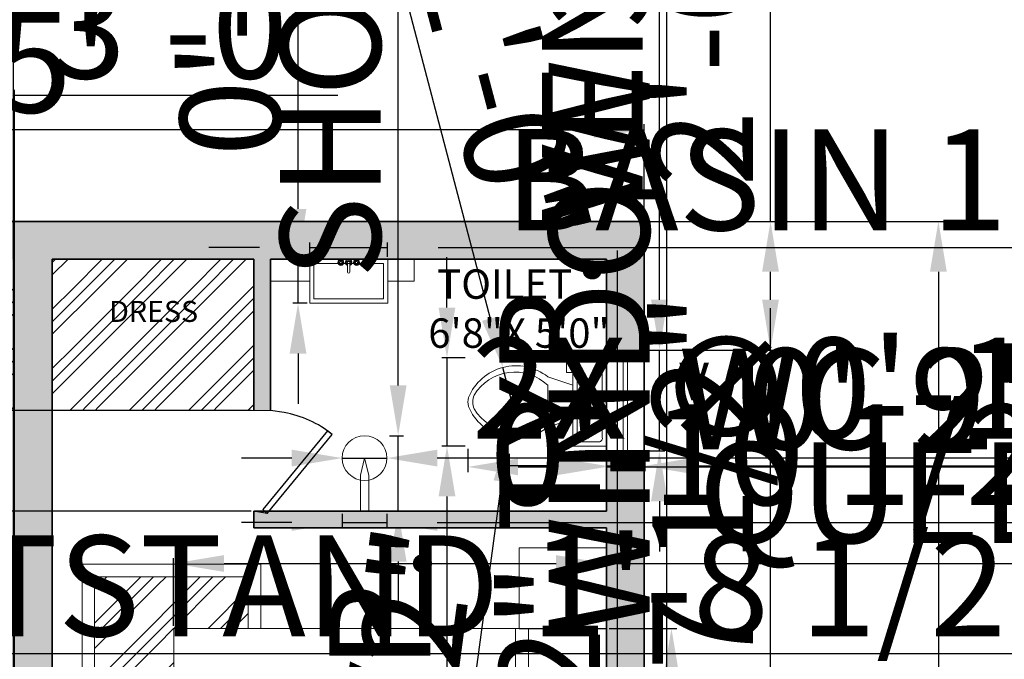
# Model space of a CAD drawing. Units: inches. Extents: x 830 to 1639, y 2591 to 3595.
# Tile 5 of 7: x 1133 to 1367, y 3108 to 3260. Entities that reach past the tile are written whole.
import ezdxf

# ---------------------------------------------------------------- set-up
doc = ezdxf.new("R2010")
doc.units = ezdxf.units.IN
doc.layers.get('0').update_dxf_attribs({"color": 250})
for name, color, linetype, lineweight in [('A-ANNO-DIMS', 2, 'Continuous', 18), ('A-ANNO-TEXT', 7, 'Continuous', 18), ('A-AREA-IDEN', 7, 'Continuous', 25), ('A-DOOR', 3, 'Continuous', 25), ('A-FLOR-CASE', 8, 'Continuous', 18), ('A-FLOR-FIXT', 8, 'Continuous', 18), ('A-FLOR-PATT', 252, 'Continuous', 13), ('A-FURN', 8, 'Continuous', 18), ('A-GLAZ', 4, 'Continuous', 18), ('A-WALL', 7, 'Continuous', 35), ('A-WALL-PATT', 5, 'Continuous', 13), ('C-PROP', 7, 'Continuous', 35)]:
    doc.layers.add(name, color=color, linetype=linetype, lineweight=lineweight)
doc.styles.get("Standard").update_dxf_attribs({"font": 'arial.ttf'})
doc.dimstyles.new('ISO-25', dxfattribs={"dimtxt": 24, "dimasz": 12, "dimexe": 1.25, "dimexo": 0.625, "dimtad": 1, "dimdec": 0, "dimlunit": 3, "dimtxsty": 'Standard', "dimcen": 2.5, "dimadec": 0, "dimazin": 0, "dimtfac": 1, "dimtdec": 0, "dimtmove": 0, "dimatfit": 3, "dimfxl": 1, "dimarcsym": 0})

# ---------------------------------------------------------------- blocks, each defined once
blk = doc.blocks.new('Toilet - top')
for p, q in [((9.5, -6), (9.5, -2)), ((-10, -8.5), (-8, -8.5)), ((-10, -9.5), (-10, -8.5)), ((-8, -8.5), (-8, -8)), ((-7, -8), (-7, -9.5)), ((-4, -8), (-6, -14)), ((4, -8), (6, -14)), ((-7, -9.5), (-10, -9.5)), ((4, -14), (-4, -14))]:
    blk.add_line(p, q)
blk.add_lwpolyline([(10.5, -8), (10.5, 0), (-10.5, 0), (-10.5, -8)], close=True)
for points in [[(-9.5, -2), (-9.5, -6)], [(8.5, -1), (-8.5, -1)], [(-8.5, -7), (8.5, -7)]]:
    blk.add_lwpolyline(points)
for centre, radius, start, end in [((-8.62, -1.88), 0.884, 81.8699, 188.1301), ((8.62, -1.88), 0.884, 351.8699, 98.1301), ((-8.62, -6.12), 0.884, 171.8699, 278.1301), ((8.62, -6.12), 0.884, 261.8699, 8.1301), ((3.52, -21.58), 12.17, 141.4691, 247.9714), ((4.2, -21.82), 11.33, 136.3677, 238.9468), ((-3.52, -21.58), 12.17, 292.0284, 38.5307), ((-4.2, -21.82), 11.33, 301.053, 43.6321), ((0, -27.88), 4, 245.7318, 294.2682), ((0, -29), 4, 254.8605, 285.1395)]:
    blk.add_arc(centre, radius, start, end)
blk = doc.blocks.new('*U9')
for p, q in [((-750, 0), (-750, -100)), ((0, 0), (0, -100))]:
    blk.add_line(p, q)
blk.add_lwpolyline([(0, 0), (-649.5, 375), (-671.4, 337.1), (-21.9, -37.9)], close=True)
blk.add_arc((0, 0), 750, 150, 180)
blk = doc.blocks.new('Faucet - Bathroom top')
for p, q in [((-4.107, 0.125), (-4.375, 0.125)), ((-3.75, 0.4788), (-3.75, 0.75)), ((-3.5, 0.482), (-3.5, 0.75)), ((-3.1461, 0.125), (-2.875, 0.125)), ((3.143, 0.125), (2.875, 0.125)), ((3.5, 0.4788), (3.5, 0.75)), ((3.75, 0.482), (3.75, 0.75)), ((4.1039, 0.125), (4.375, 0.125)), ((-4.1039, -0.125), (-4.375, -0.125)), ((-3.75, -0.4821), (-3.75, -0.75)), ((-3.5, -0.4789), (-3.5, -0.75)), ((-3.143, -0.125), (-2.875, -0.125)), ((-0.5, -0.8639), (-0.5, -4.5)), ((0.5, -4.5), (0.5, -0.8631)), ((3.1461, -0.125), (2.875, -0.125)), ((3.5, -0.4821), (3.5, -0.75)), ((3.75, -0.4789), (3.75, -0.75)), ((4.107, -0.125), (4.375, -0.125))]:
    blk.add_line(p, q)
for centre, radius in [((-3.625, 0), 1.375), ((-4.625, 0), 0.2795), ((-3.625, 0), 0.5), ((-3.625, 1), 0.2795), ((-2.625, 0), 0.2795), ((0, 0), 0.5), ((3.625, 0), 1.375), ((2.625, 0), 0.2795), ((3.625, 0), 0.5), ((3.625, 1), 0.2795), ((4.625, 0), 0.2795), ((-3.625, -1), 0.2795), ((3.625, -1), 0.2795)]:
    blk.add_circle(centre, radius)
for centre, radius, start, end in [((-3.625, 0), 1, 105.2407, 164.2093), ((-3.625, 0), 1, 16.44125, 74.07887), ((0, 0), 1.5, 289.6514, 250.3603), ((0, 0), 1, 300.3431, 239.7554), ((3.625, 0), 1, 106.12, 164.0884), ((3.625, 0), 1, 16.23422, 73.90469), ((-3.625, 0), 1, 196.2342, 253.9047), ((-3.625, 0), 1, 286.12, 344.0884), ((0, -4.5), 0.5, 180, 0), ((3.625, 0), 1, 196.4413, 254.0789), ((3.625, 0), 1, 285.2407, 344.2093)]:
    blk.add_arc(centre, radius, start, end)
blk = doc.blocks.new('Bed - Queen')
for p, q in [((0, -80.00003), (0, 0)), ((0, 0), (59.99999, 0)), ((59.99999, 0), (59.99999, -80.00003)), ((7.99999, -1.2), (28.79998, -1.2)), ((7.99999, -14.4), (7.99999, -1.2)), ((28.79998, -1.2), (28.79998, -14.4)), ((31.19999, -1.2), (51.99999, -1.2)), ((31.19999, -14.4), (31.19999, -1.2)), ((51.99999, -1.2), (51.99999, -16.4)), ((0, -14.4), (44.8, -14.4)), ((59.99999, -29.6), (44.8, -14.4)), ((44.8, -14.4), (44.8, -29.6)), ((44.8, -16.8), (0, -16.8)), ((51.99999, -16.4), (46.79936, -16.4)), ((44.8, -29.6), (59.99999, -29.6)), ((59.99999, -80.00003), (0, -80.00003))]:
    blk.add_line(p, q)
blk = doc.blocks.new('*D14')
at = {"layer": 'A-ANNO-DIMS', "color": 0, "lineweight": -2, "transparency": 16777216}
for p, q in [((1282.21, 3212.09), (1352.88, 3212.09)), ((1351.63, 3200.09), (1351.63, 2684.09)), ((1282.21, 2672.09), (1352.88, 2672.09))]:
    blk.add_line(p, q, dxfattribs=at)
at = {"layer": 'A-ANNO-DIMS', "color": 0, "transparency": 16777216}
for points in [[(1349.63, 3200.09), (1353.63, 3200.09), (1351.63, 3212.09)], [(1349.63, 2684.09), (1353.63, 2684.09), (1351.63, 2672.09)]]:
    blk.add_solid(points, dxfattribs=at)
at = {"layer": 'Defpoints', "color": 0, "transparency": 16777216}
for p in [(1281.59, 3212.09), (1281.59, 2672.09), (1351.63, 2672.09)]:
    blk.add_point(p, dxfattribs=at)
at = {"layer": 'A-ANNO-DIMS', "color": 0, "transparency": 16777216, "insert": (1338.8, 2942.09), "char_height": 24, "attachment_point": 5, "rotation": 90}
blk.add_mtext("45'", dxfattribs=at)
blk = doc.blocks.new('*D15')
at = {"layer": 'A-ANNO-DIMS', "color": 0, "lineweight": -2, "transparency": 16777216}
for p, q in [((981.59, 3212.71), (981.59, 3235.25)), ((993.59, 3234), (1269.59, 3234)), ((1281.59, 3212.71), (1281.59, 3235.25))]:
    blk.add_line(p, q, dxfattribs=at)
at = {"layer": 'A-ANNO-DIMS', "color": 0, "transparency": 16777216}
for points in [[(993.59, 3236), (993.59, 3232), (981.59, 3234)], [(1269.59, 3236), (1269.59, 3232), (1281.59, 3234)]]:
    blk.add_solid(points, dxfattribs=at)
at = {"layer": 'Defpoints', "color": 0, "transparency": 16777216}
for p in [(1281.59, 3234), (981.59, 3212.09), (1281.59, 3212.09)]:
    blk.add_point(p, dxfattribs=at)
at = {"layer": 'A-ANNO-DIMS', "color": 0, "transparency": 16777216, "insert": (1131.59, 3246.88), "char_height": 24, "attachment_point": 5}
blk.add_mtext("25'", dxfattribs=at)
blk = doc.blocks.new('VENT-24IN')
for p, q in [((0, 24), (9, 24)), ((0, 0), (0, 24)), ((4, 0), (4, 24)), ((5, 24), (5, 0)), ((9, 24), (9, 0)), ((9, 0), (0, 0))]:
    blk.add_line(p, q)
blk = doc.blocks.new('BEDSIDE-TABLE')
blk.add_lwpolyline([(20.72, 0), (0, 0), (0, 19.25), (20.72, 19.25)], close=True)
blk = doc.blocks.new('LAVATORY-RECT')
for points in [[(0, 10.45), (18.57, 10.45), (18.57, 0), (0, 0)], [(1, 9.45), (17.57, 9.45), (17.57, 1), (1, 1)]]:
    blk.add_lwpolyline(points, close=True)
blk = doc.blocks.new('SHOWER-HEAD-PLAN')
for p, q in [((4.38, 8.59), (5.33, 12.63)), ((5.33, 12.63), (6.38, 8.59)), ((4.38, 0), (4.38, 8.59)), ((6.38, 0), (6.38, 8.59))]:
    blk.add_line(p, q)
blk.add_circle((5.33, 12.63), 5.33)
blk = doc.blocks.new('BED-RUG-PLAN')
for points in [[(0, 92.63), (0, 105.69), (42.59, 105.69), (42.59, 0), (0, 0), (0, 15.31)], [(3, 92.63), (3, 102.69), (39.59, 102.69), (39.59, 3), (3, 3), (3, 15.31)]]:
    blk.add_lwpolyline(points)
blk = doc.blocks.new('*D22')
at = {"layer": 'A-ANNO-DIMS', "color": 0, "lineweight": -2, "transparency": 16777216}
for p, q in [((1286.99, 3094.42), (1286.99, 3411.37)), ((1282.21, 3094.42), (1288.24, 3094.42)), ((1286.99, 3070.42), (1286.99, 3082.42)), ((1282.21, 3058.42), (1288.24, 3058.42))]:
    blk.add_line(p, q, dxfattribs=at)
at = {"layer": 'A-ANNO-DIMS', "color": 0, "transparency": 16777216}
for points in [[(1284.99, 3082.42), (1288.99, 3082.42), (1286.99, 3094.42)], [(1284.99, 3070.42), (1288.99, 3070.42), (1286.99, 3058.42)]]:
    blk.add_solid(points, dxfattribs=at)
at = {"layer": 'Defpoints', "color": 0, "transparency": 16777216}
for p in [(1281.59, 3094.42), (1286.99, 3094.42), (1281.59, 3058.42)]:
    blk.add_point(p, dxfattribs=at)
at = {"layer": 'A-ANNO-DIMS', "color": 0, "transparency": 16777216, "insert": (1273.94, 3258.89), "char_height": 24, "attachment_point": 5, "rotation": 90}
blk.add_mtext('WINDOW 3\'-0" TYP.', dxfattribs=at)
blk = doc.blocks.new('*D24')
at = {"layer": 'A-ANNO-DIMS', "color": 0, "lineweight": -2, "transparency": 16777216}
for p, q in [((1285.19, 3193.45), (1285.19, 3452.97)), ((1282.21, 3181.45), (1286.44, 3181.45)), ((1285.19, 3157.45), (1285.19, 3181.45)), ((1282.21, 3157.45), (1286.44, 3157.45)), ((1285.19, 3145.45), (1285.19, 3133.45))]:
    blk.add_line(p, q, dxfattribs=at)
at = {"layer": 'A-ANNO-DIMS', "color": 0, "transparency": 16777216}
for points in [[(1283.19, 3193.45), (1287.19, 3193.45), (1285.19, 3181.45)], [(1283.19, 3145.45), (1287.19, 3145.45), (1285.19, 3157.45)]]:
    blk.add_solid(points, dxfattribs=at)
at = {"layer": 'Defpoints', "color": 0, "transparency": 16777216}
for p in [(1281.59, 3181.45), (1285.19, 3181.45), (1281.59, 3157.45)]:
    blk.add_point(p, dxfattribs=at)
at = {"layer": 'A-ANNO-DIMS', "color": 0, "transparency": 16777216, "insert": (1272.31, 3329.21), "char_height": 24, "attachment_point": 5, "rotation": 90}
blk.add_mtext('VENT 2\'-0" TYP.', dxfattribs=at)
blk = doc.blocks.new('*D25')
at = {"layer": 'A-ANNO-DIMS', "color": 0, "lineweight": -2, "transparency": 16777216}
for p, q in [((1272.59, 3156.83), (1272.59, 3152.6)), ((1281.59, 3156.83), (1281.59, 3152.6)), ((1260.59, 3153.85), (1248.59, 3153.85)), ((1272.59, 3153.85), (1281.59, 3153.85)), ((1293.59, 3153.85), (1453.13, 3153.85))]:
    blk.add_line(p, q, dxfattribs=at)
at = {"layer": 'A-ANNO-DIMS', "color": 0, "transparency": 16777216}
for points in [[(1260.59, 3155.85), (1260.59, 3151.85), (1272.59, 3153.85)], [(1293.59, 3155.85), (1293.59, 3151.85), (1281.59, 3153.85)]]:
    blk.add_solid(points, dxfattribs=at)
at = {"layer": 'Defpoints', "color": 0, "transparency": 16777216}
for p in [(1272.59, 3157.45), (1281.59, 3157.45), (1281.59, 3153.85)]:
    blk.add_point(p, dxfattribs=at)
at = {"layer": 'A-ANNO-DIMS', "color": 0, "transparency": 16777216, "insert": (1379.36, 3166.73), "char_height": 24, "attachment_point": 5}
blk.add_mtext('0\'-9" TYP.', dxfattribs=at)
blk = doc.blocks.new('*D26')
at = {"layer": 'A-ANNO-DIMS', "color": 0, "lineweight": -2, "transparency": 16777216}
for p, q in [((990.59, 3111.63), (990.59, 3107.9)), ((1011.31, 3111.63), (1011.31, 3107.9)), ((978.59, 3109.15), (966.59, 3109.15)), ((990.59, 3109.15), (1011.31, 3109.15)), ((1023.31, 3109.15), (1464.86, 3109.15))]:
    blk.add_line(p, q, dxfattribs=at)
at = {"layer": 'A-ANNO-DIMS', "color": 0, "transparency": 16777216}
for points in [[(978.59, 3111.15), (978.59, 3107.15), (990.59, 3109.15)], [(1023.31, 3111.15), (1023.31, 3107.15), (1011.31, 3109.15)]]:
    blk.add_solid(points, dxfattribs=at)
at = {"layer": 'Defpoints', "color": 0, "transparency": 16777216}
for p in [(990.59, 3112.26), (1011.31, 3112.26), (1011.31, 3109.15)]:
    blk.add_point(p, dxfattribs=at)
at = {"layer": 'A-ANNO-DIMS', "color": 0, "transparency": 16777216, "insert": (1250.08, 3122.18), "char_height": 24, "attachment_point": 5}
blk.add_mtext('NIGHTSTAND 1\'-8 1/2" TYP.', dxfattribs=at)
blk = doc.blocks.new('*D29')
at = {"layer": 'A-ANNO-DIMS', "color": 0, "lineweight": -2, "transparency": 16777216}
for p, q in [((1275.17, 2989.75), (1275.17, 3205.2)), ((1263.19, 2989.75), (1276.42, 2989.75)), ((1275.17, 2965.09), (1275.17, 2977.75)), ((1263.19, 2953.09), (1276.42, 2953.09))]:
    blk.add_line(p, q, dxfattribs=at)
at = {"layer": 'A-ANNO-DIMS', "color": 0, "transparency": 16777216}
for points in [[(1273.17, 2977.75), (1277.17, 2977.75), (1275.17, 2989.75)], [(1273.17, 2965.09), (1277.17, 2965.09), (1275.17, 2953.09)]]:
    blk.add_solid(points, dxfattribs=at)
at = {"layer": 'Defpoints', "color": 0, "transparency": 16777216}
for p in [(1262.57, 2989.75), (1275.17, 2989.75), (1262.57, 2953.09)]:
    blk.add_point(p, dxfattribs=at)
at = {"layer": 'A-ANNO-DIMS', "color": 0, "transparency": 16777216, "insert": (1262.13, 3103.48), "char_height": 24, "attachment_point": 5, "rotation": 90}
blk.add_mtext('3\'-0 1/2" TYP.', dxfattribs=at)
blk = doc.blocks.new('*D30')
at = {"layer": 'A-ANNO-DIMS', "color": 0, "lineweight": -2, "transparency": 16777216}
for p, q in [((1239.54, 3157.95), (1239.54, 3152.37)), ((1272.59, 3157.95), (1272.59, 3152.37)), ((1251.54, 3153.62), (1260.59, 3153.62)), ((1272.59, 3153.62), (1498.29, 3153.62))]:
    blk.add_line(p, q, dxfattribs=at)
at = {"layer": 'A-ANNO-DIMS', "color": 0, "transparency": 16777216}
for points in [[(1251.54, 3155.62), (1251.54, 3151.62), (1239.54, 3153.62)], [(1260.59, 3155.62), (1260.59, 3151.62), (1272.59, 3153.62)]]:
    blk.add_solid(points, dxfattribs=at)
at = {"layer": 'Defpoints', "color": 0, "transparency": 16777216}
for p in [(1239.54, 3158.58), (1272.59, 3158.58), (1272.59, 3153.62)]:
    blk.add_point(p, dxfattribs=at)
at = {"layer": 'A-ANNO-DIMS', "color": 0, "transparency": 16777216, "insert": (1391.44, 3166.66), "char_height": 24, "attachment_point": 5}
blk.add_mtext('WC 2\'-9" TYP.', dxfattribs=at)
blk = doc.blocks.new('*D31')
at = {"layer": 'A-ANNO-DIMS', "color": 0, "lineweight": -2, "transparency": 16777216}
for p, q in [((1234.59, 3191.58), (1234.59, 3203.58)), ((1238.92, 3179.58), (1233.34, 3179.58)), ((1234.59, 3179.58), (1234.59, 3158.58)), ((1238.92, 3158.58), (1233.34, 3158.58)), ((1234.59, 3146.58), (1234.59, 2989.29))]:
    blk.add_line(p, q, dxfattribs=at)
at = {"layer": 'A-ANNO-DIMS', "color": 0, "transparency": 16777216}
for points in [[(1232.59, 3191.58), (1236.59, 3191.58), (1234.59, 3179.58)], [(1232.59, 3146.58), (1236.59, 3146.58), (1234.59, 3158.58)]]:
    blk.add_solid(points, dxfattribs=at)
at = {"layer": 'Defpoints', "color": 0, "transparency": 16777216}
for p in [(1239.54, 3179.58), (1234.59, 3158.58), (1239.54, 3158.58)]:
    blk.add_point(p, dxfattribs=at)
at = {"layer": 'A-ANNO-DIMS', "color": 0, "transparency": 16777216, "insert": (1221.71, 3061.94), "char_height": 24, "attachment_point": 5, "rotation": 90}
blk.add_mtext('1\'-9" TYP.', dxfattribs=at)
blk = doc.blocks.new('*D34')
at = {"layer": 'A-ANNO-DIMS', "color": 0, "lineweight": -2, "transparency": 16777216}
for p, q in [((1189.9, 3205.85), (1177.9, 3205.85)), ((1201.9, 3203.69), (1201.9, 3207.1)), ((1201.9, 3205.85), (1220.46, 3205.85)), ((1220.46, 3203.69), (1220.46, 3207.1)), ((1232.46, 3205.85), (1556.8, 3205.85))]:
    blk.add_line(p, q, dxfattribs=at)
at = {"layer": 'A-ANNO-DIMS', "color": 0, "transparency": 16777216}
for points in [[(1189.9, 3207.85), (1189.9, 3203.85), (1201.9, 3205.85)], [(1232.46, 3207.85), (1232.46, 3203.85), (1220.46, 3205.85)]]:
    blk.add_solid(points, dxfattribs=at)
at = {"layer": 'Defpoints', "color": 0, "transparency": 16777216}
for p in [(1220.46, 3205.85), (1201.9, 3203.07), (1220.46, 3203.07)]:
    blk.add_point(p, dxfattribs=at)
at = {"layer": 'A-ANNO-DIMS', "color": 0, "transparency": 16777216, "insert": (1400.63, 3218.88), "char_height": 24, "attachment_point": 5}
blk.add_mtext('BASIN 1\'-6 1/2" TYP.', dxfattribs=at)
blk = doc.blocks.new('*D35')
at = {"layer": 'A-ANNO-DIMS', "color": 0, "lineweight": -2, "transparency": 16777216}
for p, q in [((1199.11, 3215.07), (1199.11, 3449.18)), ((1201.27, 3203.07), (1197.86, 3203.07)), ((1199.11, 3192.62), (1199.11, 3203.07)), ((1201.27, 3192.62), (1197.86, 3192.62)), ((1199.11, 3180.62), (1199.11, 3168.62))]:
    blk.add_line(p, q, dxfattribs=at)
at = {"layer": 'A-ANNO-DIMS', "color": 0, "transparency": 16777216}
for points in [[(1197.11, 3215.07), (1201.11, 3215.07), (1199.11, 3203.07)], [(1197.11, 3180.62), (1201.11, 3180.62), (1199.11, 3192.62)]]:
    blk.add_solid(points, dxfattribs=at)
at = {"layer": 'Defpoints', "color": 0, "transparency": 16777216}
for p in [(1199.11, 3203.07), (1201.9, 3203.07), (1201.9, 3192.62)]:
    blk.add_point(p, dxfattribs=at)
at = {"layer": 'A-ANNO-DIMS', "color": 0, "transparency": 16777216, "insert": (1186.08, 3338.12), "char_height": 24, "attachment_point": 5, "rotation": 90}
blk.add_mtext('0\'-10 1/2" TYP.', dxfattribs=at)
blk = doc.blocks.new('*D36')
at = {"layer": 'A-ANNO-DIMS', "color": 0, "lineweight": -2, "transparency": 16777216}
for p, q in [((1169.49, 3115.77), (1169.49, 3131.86)), ((1272.59, 3115.77), (1272.59, 3131.86)), ((1181.49, 3130.61), (1260.59, 3130.61)), ((1272.59, 3130.61), (1638.88, 3130.61))]:
    blk.add_line(p, q, dxfattribs=at)
at = {"layer": 'A-ANNO-DIMS', "color": 0, "transparency": 16777216}
for points in [[(1181.49, 3132.61), (1181.49, 3128.61), (1169.49, 3130.61)], [(1260.59, 3132.61), (1260.59, 3128.61), (1272.59, 3130.61)]]:
    blk.add_solid(points, dxfattribs=at)
at = {"layer": 'Defpoints', "color": 0, "transparency": 16777216}
for p in [(1272.59, 3130.61), (1169.49, 3115.15), (1272.59, 3115.15)]:
    blk.add_point(p, dxfattribs=at)
at = {"layer": 'A-ANNO-DIMS', "color": 0, "transparency": 16777216, "insert": (1461.74, 3144.38), "char_height": 24, "attachment_point": 5}
blk.add_mtext('QUEEN BED 8\'-7" TYP.', dxfattribs=at)
blk = doc.blocks.new('*D37')
at = {"layer": 'A-ANNO-DIMS', "color": 0, "lineweight": -2, "transparency": 16777216}
for p, q in [((1273.21, 3115.15), (1289.3, 3115.15)), ((1288.05, 3103.15), (1288.05, 3049.83)), ((1273.21, 3037.83), (1289.3, 3037.83)), ((1288.05, 3037.83), (1288.05, 2822.23))]:
    blk.add_line(p, q, dxfattribs=at)
at = {"layer": 'A-ANNO-DIMS', "color": 0, "transparency": 16777216}
for points in [[(1286.05, 3103.15), (1290.05, 3103.15), (1288.05, 3115.15)], [(1286.05, 3049.83), (1290.05, 3049.83), (1288.05, 3037.83)]]:
    blk.add_solid(points, dxfattribs=at)
at = {"layer": 'Defpoints', "color": 0, "transparency": 16777216}
for p in [(1272.59, 3115.15), (1272.59, 3037.83), (1288.05, 3037.83)]:
    blk.add_point(p, dxfattribs=at)
at = {"layer": 'A-ANNO-DIMS', "color": 0, "transparency": 16777216, "insert": (1275.02, 2924.03), "char_height": 24, "attachment_point": 5, "rotation": 90}
blk.add_mtext('6\'-5 1/2" TYP.', dxfattribs=at)
blk = doc.blocks.new('*D38')
at = {"layer": 'A-ANNO-DIMS', "color": 0, "lineweight": -2, "transparency": 16777216}
for p, q in [((1222.96, 3173.04), (1222.96, 3595.13)), ((1220.89, 3161.04), (1224.21, 3161.04)), ((1222.96, 3143.09), (1222.96, 3161.04)), ((1220.89, 3143.09), (1224.21, 3143.09)), ((1222.96, 3131.09), (1222.96, 3119.09))]:
    blk.add_line(p, q, dxfattribs=at)
at = {"layer": 'A-ANNO-DIMS', "color": 0, "transparency": 16777216}
for points in [[(1220.96, 3173.04), (1224.96, 3173.04), (1222.96, 3161.04)], [(1220.96, 3131.09), (1224.96, 3131.09), (1222.96, 3143.09)]]:
    blk.add_solid(points, dxfattribs=at)
at = {"layer": 'Defpoints', "color": 0, "transparency": 16777216}
for p in [(1220.27, 3161.04), (1222.96, 3161.04), (1220.27, 3143.09)]:
    blk.add_point(p, dxfattribs=at)
at = {"layer": 'A-ANNO-DIMS', "color": 0, "transparency": 16777216, "insert": (1209.92, 3390.09), "char_height": 24, "attachment_point": 5, "rotation": 90}
blk.add_mtext('SHOWER HEAD 1\'-6" TYP.', dxfattribs=at)
blk = doc.blocks.new('*D39')
at = {"layer": 'A-ANNO-DIMS', "color": 0, "lineweight": -2, "transparency": 16777216}
for p, q in [((1209.62, 3142.46), (1209.62, 3139.14)), ((1220.27, 3142.46), (1220.27, 3139.14)), ((1197.62, 3140.39), (1185.62, 3140.39)), ((1209.62, 3140.39), (1220.27, 3140.39)), ((1232.27, 3140.39), (1466.38, 3140.39))]:
    blk.add_line(p, q, dxfattribs=at)
at = {"layer": 'A-ANNO-DIMS', "color": 0, "transparency": 16777216}
for points in [[(1197.62, 3142.39), (1197.62, 3138.39), (1209.62, 3140.39)], [(1232.27, 3142.39), (1232.27, 3138.39), (1220.27, 3140.39)]]:
    blk.add_solid(points, dxfattribs=at)
at = {"layer": 'Defpoints', "color": 0, "transparency": 16777216}
for p in [(1209.62, 3143.09), (1220.27, 3143.09), (1220.27, 3140.39)]:
    blk.add_point(p, dxfattribs=at)
at = {"layer": 'A-ANNO-DIMS', "color": 0, "transparency": 16777216, "insert": (1355.32, 3153.43), "char_height": 24, "attachment_point": 5}
blk.add_mtext('0\'-10 1/2" TYP.', dxfattribs=at)
blk = doc.blocks.new('*D40')
at = {"layer": 'A-ANNO-DIMS', "color": 0, "lineweight": -2, "transparency": 16777216}
for p, q in [((1131.38, 3125.32), (1131.38, 3423.36)), ((1116.15, 3125.32), (1132.63, 3125.32)), ((1131.38, 3031.63), (1131.38, 3113.32)), ((1116.15, 3019.63), (1132.63, 3019.63))]:
    blk.add_line(p, q, dxfattribs=at)
at = {"layer": 'A-ANNO-DIMS', "color": 0, "transparency": 16777216}
for points in [[(1129.38, 3113.32), (1133.38, 3113.32), (1131.38, 3125.32)], [(1129.38, 3031.63), (1133.38, 3031.63), (1131.38, 3019.63)]]:
    blk.add_solid(points, dxfattribs=at)
at = {"layer": 'Defpoints', "color": 0, "transparency": 16777216}
for p in [(1115.52, 3125.32), (1131.38, 3125.32), (1115.52, 3019.63)]:
    blk.add_point(p, dxfattribs=at)
at = {"layer": 'A-ANNO-DIMS', "color": 0, "transparency": 16777216, "insert": (1118.34, 3280.34), "char_height": 24, "attachment_point": 5, "rotation": 90}
blk.add_mtext('RUG 8\'-9 1/2" TYP.', dxfattribs=at)
blk = doc.blocks.new('*D49')
at = {"layer": 'A-ANNO-DIMS', "color": 0, "lineweight": -2, "transparency": 16777216}
for p, q in [((1095.59, 2991.71), (1095.59, 3243.39)), ((1131.59, 2992.51), (1131.59, 3243.39)), ((1107.59, 3242.14), (1119.59, 3242.14)), ((1131.59, 3242.14), (1208.62, 3242.14))]:
    blk.add_line(p, q, dxfattribs=at)
at = {"layer": 'A-ANNO-DIMS', "color": 0, "transparency": 16777216}
for points in [[(1107.59, 3244.14), (1107.59, 3240.14), (1095.59, 3242.14)], [(1119.59, 3244.14), (1119.59, 3240.14), (1131.59, 3242.14)]]:
    blk.add_solid(points, dxfattribs=at)
at = {"layer": 'Defpoints', "color": 0, "transparency": 16777216}
for p in [(1131.59, 3242.14), (1095.59, 2991.09), (1131.59, 2991.89)]:
    blk.add_point(p, dxfattribs=at)
at = {"layer": 'A-ANNO-DIMS', "color": 0, "transparency": 16777216, "insert": (1176.11, 3255.02), "char_height": 24, "attachment_point": 5}
blk.add_mtext('3\'-0"', dxfattribs=at)
blk = doc.blocks.new('*D50')
at = {"layer": 'A-ANNO-DIMS', "color": 0, "lineweight": -2, "transparency": 16777216}
for p, q in [((951.54, 3179.09), (951.54, 3256.54)), ((1187.96, 3167.09), (950.29, 3167.09)), ((951.54, 3143.09), (951.54, 3167.09)), ((1187.96, 3143.09), (950.29, 3143.09)), ((951.54, 3131.09), (951.54, 3119.09))]:
    blk.add_line(p, q, dxfattribs=at)
at = {"layer": 'A-ANNO-DIMS', "color": 0, "transparency": 16777216}
for points in [[(949.54, 3179.09), (953.54, 3179.09), (951.54, 3167.09)], [(949.54, 3131.09), (953.54, 3131.09), (951.54, 3143.09)]]:
    blk.add_solid(points, dxfattribs=at)
at = {"layer": 'Defpoints', "color": 0, "transparency": 16777216}
for p in [(951.54, 3167.09), (1188.59, 3167.09), (1188.59, 3143.09)]:
    blk.add_point(p, dxfattribs=at)
at = {"layer": 'A-ANNO-DIMS', "color": 0, "transparency": 16777216, "insert": (938.66, 3223.82), "char_height": 24, "attachment_point": 5, "rotation": 90}
blk.add_mtext('2\'-0"', dxfattribs=at)
blk = doc.blocks.new('*D68')
at = {"layer": 'A-ANNO-DIMS', "color": 0, "lineweight": -2, "transparency": 16777216}
for p, q in [((1311.64, 3058.42), (1311.64, 3191.39)), ((1273.21, 3058.42), (1312.89, 3058.42)), ((1311.64, 3003.09), (1311.64, 3046.42)), ((1273.21, 2991.09), (1312.89, 2991.09))]:
    blk.add_line(p, q, dxfattribs=at)
at = {"layer": 'A-ANNO-DIMS', "color": 0, "transparency": 16777216}
for points in [[(1309.64, 3046.42), (1313.64, 3046.42), (1311.64, 3058.42)], [(1309.64, 3003.09), (1313.64, 3003.09), (1311.64, 2991.09)]]:
    blk.add_solid(points, dxfattribs=at)
at = {"layer": 'Defpoints', "color": 0, "transparency": 16777216}
for p in [(1272.59, 3058.42), (1311.64, 3058.42), (1272.59, 2991.09)]:
    blk.add_point(p, dxfattribs=at)
at = {"layer": 'A-ANNO-DIMS', "color": 0, "transparency": 16777216, "insert": (1298.61, 3130.9), "char_height": 24, "attachment_point": 5, "rotation": 90}
blk.add_mtext('5\'-7 1/2"', dxfattribs=at)
blk = doc.blocks.new('*D70')
at = {"layer": 'A-ANNO-DIMS', "color": 0, "lineweight": -2, "transparency": 16777216}
for p, q in [((1311.64, 3212.09), (1311.64, 3345.47)), ((1282.21, 3212.09), (1312.89, 3212.09)), ((1311.64, 3193.45), (1311.64, 3200.09)), ((1282.21, 3181.45), (1312.89, 3181.45))]:
    blk.add_line(p, q, dxfattribs=at)
at = {"layer": 'A-ANNO-DIMS', "color": 0, "transparency": 16777216}
for points in [[(1309.64, 3200.09), (1313.64, 3200.09), (1311.64, 3212.09)], [(1309.64, 3193.45), (1313.64, 3193.45), (1311.64, 3181.45)]]:
    blk.add_solid(points, dxfattribs=at)
at = {"layer": 'Defpoints', "color": 0, "transparency": 16777216}
for p in [(1281.59, 3212.09), (1311.64, 3212.09), (1281.59, 3181.45)]:
    blk.add_point(p, dxfattribs=at)
at = {"layer": 'A-ANNO-DIMS', "color": 0, "transparency": 16777216, "insert": (1298.61, 3284.78), "char_height": 24, "attachment_point": 5, "rotation": 90}
blk.add_mtext('2\'-6 1/2"', dxfattribs=at)
blk = doc.blocks.new('*D75')
at = {"layer": 'A-ANNO-DIMS', "color": 0, "lineweight": -2, "transparency": 16777216}
for p, q in [((1206.32, 3335.67), (1244.87, 3188.93)), ((1251.01, 3165.56), (1247.92, 3177.33))]:
    blk.add_line(p, q, dxfattribs=at)
at = {"layer": 'A-ANNO-DIMS', "color": 0, "transparency": 16777216}
blk.add_solid([(1246.8, 3189.44), (1242.93, 3188.43), (1247.92, 3177.33)], dxfattribs=at)
at = {"layer": 'Defpoints', "color": 0, "transparency": 16777216}
for p in [(1247.92, 3177.33), (1251.01, 3165.56)]:
    blk.add_point(p, dxfattribs=at)
at = {"layer": 'A-ANNO-DIMS', "color": 0, "transparency": 16777216, "insert": (1236.52, 3271.38), "char_height": 24, "attachment_point": 5, "rotation": 284.7203}
blk.add_mtext('6X R1\'-0"', dxfattribs=at)
blk = doc.blocks.new('*D76')
at = {"layer": 'A-ANNO-DIMS', "color": 0, "lineweight": -2, "transparency": 16777216}
for p, q in [((1250.77, 3173.28), (1249.26, 3162.05)), ((1217.52, 2925.89), (1247.66, 3150.16))]:
    blk.add_line(p, q, dxfattribs=at)
at = {"layer": 'A-ANNO-DIMS', "color": 0, "transparency": 16777216}
blk.add_solid([(1245.68, 3150.42), (1249.65, 3149.89), (1249.26, 3162.05)], dxfattribs=at)
at = {"layer": 'Defpoints', "color": 0, "transparency": 16777216}
for p in [(1250.77, 3173.28), (1249.26, 3162.05)]:
    blk.add_point(p, dxfattribs=at)
at = {"layer": 'A-ANNO-DIMS', "color": 0, "transparency": 16777216, "insert": (1218.87, 3033.81), "char_height": 24, "attachment_point": 5, "rotation": 82.3443}
blk.add_mtext('6X R0\'-11 1/2"', dxfattribs=at)
blk = doc.blocks.new('*D77')
at = {"layer": 'A-ANNO-DIMS', "color": 0, "lineweight": -2, "transparency": 16777216}
for p, q in [((1197.62, 3155.72), (1185.62, 3155.72)), ((1209.62, 3155.72), (1220.27, 3155.72)), ((1460.7, 3155.7), (1232.27, 3155.72))]:
    blk.add_line(p, q, dxfattribs=at)
at = {"layer": 'A-ANNO-DIMS', "color": 0, "transparency": 16777216}
for points in [[(1197.62, 3157.72), (1197.62, 3153.72), (1209.62, 3155.72)], [(1232.27, 3157.72), (1232.27, 3153.72), (1220.27, 3155.72)]]:
    blk.add_solid(points, dxfattribs=at)
at = {"layer": 'Defpoints', "color": 0, "transparency": 16777216}
for p in [(1209.62, 3155.72), (1220.27, 3155.72)]:
    blk.add_point(p, dxfattribs=at)
at = {"layer": 'A-ANNO-DIMS', "color": 0, "transparency": 16777216, "insert": (1352.48, 3169.26), "char_height": 24, "attachment_point": 5, "rotation": 359.9951}
blk.add_mtext('2X ∅0\'-10 1/2"', dxfattribs=at)

msp = doc.modelspace()

# ---------------------------------------------------------------- hatches: boundary and pattern name
at = {"layer": 'A-FLOR-PATT'}
h = msp.add_hatch(dxfattribs=at)
h.set_pattern_fill('GOST_GROUND', color=256)
h.paths.add_polyline_path([(1112.52, 3122.32), (1075.93, 3122.32), (1075.93, 3112.26), (1093.69, 3112.26), (1093.69, 3034.94), (1075.93, 3034.94), (1075.93, 3022.63), (1112.52, 3022.63)])
h.paths.add_polyline_path([(1169.49, 3115.15), (1187.25, 3115.15), (1187.25, 3127.45), (1150.65, 3127.45), (1150.65, 3027.77), (1187.25, 3027.77), (1187.25, 3037.83), (1169.49, 3037.83)])
h.paths.add_polyline_path([(1131.59, 3203.09), (1083.59, 3203.09), (1083.59, 3167.09), (1131.59, 3167.09)])
h.paths.add_polyline_path([(1188.59, 3203.09), (1140.59, 3203.09), (1140.59, 3167.09), (1188.59, 3167.09)])
at = {"layer": 'A-WALL-PATT'}
h = msp.add_hatch(color=256, dxfattribs=at)
h.dxf.hatch_style = 1
h.paths.add_polyline_path([(990.59, 3203.09), (1079.59, 3203.09), (1079.59, 3167.09), (1083.59, 3167.09), (1083.59, 3203.09), (1131.59, 3203.09), (1131.59, 2987.09), (1140.59, 2987.09), (1140.59, 2991.89), (1140.59, 3203.09), (1188.59, 3203.09), (1188.59, 3167.09), (1192.59, 3167.09), (1192.59, 3203.09), (1272.59, 3203.09), (1272.59, 3181.45), (1281.59, 3181.45), (1281.59, 3212.09), (981.59, 3212.09), (981.59, 3182.32), (990.59, 3182.32)])
h = msp.add_hatch(color=256, dxfattribs=at)
h.dxf.hatch_style = 1
h.paths.add_polyline_path([(1272.59, 3143.09), (1192.23, 3143.09), (1191.79, 3142.55), (1188.59, 3143.09), (1188.59, 3139.09), (1272.59, 3139.09), (1272.59, 3094.42), (1281.59, 3094.42), (1281.59, 3157.45), (1272.59, 3157.45)])

# ---------------------------------------------------------------- linework, layer by layer
at = {"layer": 'A-FLOR-CASE'}
for p, q in [((1226.8, 3197.84), (1226.8, 3203.09)), ((1201.9, 3197.84), (1192.59, 3197.84)), ((1220.46, 3197.84), (1226.8, 3197.84)), ((1140.59, 3167.09), (1192.59, 3167.09))]:
    msp.add_line(p, q, dxfattribs=at)
at = {"layer": 'A-WALL'}
for p, q in [((1140.59, 2991.09), (1140.59, 3203.09)), ((1140.59, 3203.09), (1188.59, 3203.09)), ((1188.59, 3167.09), (1188.59, 3203.09)), ((1192.59, 3167.09), (1192.59, 3203.09)), ((1192.59, 3203.09), (1272.59, 3203.09)), ((1272.59, 3203.09), (1272.59, 3143.09)), ((1272.59, 3143.09), (1272.59, 3203.09)), ((1188.59, 3143.09), (1272.59, 3143.09)), ((1188.59, 3139.09), (1188.59, 3143.09)), ((1140.59, 2987.09), (1140.59, 3139.09)), ((1188.59, 3139.09), (1272.59, 3139.09)), ((1272.59, 3139.09), (1272.59, 2991.09)), ((1272.59, 2991.09), (1272.59, 3139.09))]:
    msp.add_line(p, q, dxfattribs=at)
at = {"layer": 'C-PROP'}
msp.add_lwpolyline([(981.59, 3212.09), (1281.59, 3212.09), (1281.59, 2672.09), (981.59, 2672.09)], close=True, dxfattribs=at)

# ---------------------------------------------------------------- block references
at = {"layer": 'A-DOOR', "xscale": 0.0324414001615905, "yscale": 0.0324414001615905, "zscale": 0.0324414001615905, "rotation": 260.5376777919744}
msp.add_blockref('*U9', (1191.79, 3142.55), dxfattribs=at)
at = {"layer": 'A-FLOR-FIXT'}
for name, p in [('LAVATORY-RECT', (1201.9, 3192.62)), ('SHOWER-HEAD-PLAN', (1209.62, 3143.09))]:
    msp.add_blockref(name, p, dxfattribs=at)
at = {"layer": 'A-FLOR-FIXT', "xscale": 0.5159985736076383, "yscale": 0.5159985736076383, "zscale": 0.5159985736076383}
msp.add_blockref('Faucet - Bathroom top', (1211.18, 3202.32), dxfattribs=at)
at = {"layer": 'A-FLOR-FIXT', "rotation": 270}
msp.add_blockref('Toilet - top', (1272.59, 3169.08), dxfattribs=at)
at = {"layer": 'A-FURN'}
msp.add_blockref('BEDSIDE-TABLE', (1251.78, 3115.08), dxfattribs=at)
at = {"layer": 'A-FURN', "rotation": 180}
msp.add_blockref('BED-RUG-PLAN', (1190.25, 3130.45), dxfattribs=at)
at = {"layer": 'A-FURN', "xscale": 1.288695656948927, "yscale": 1.288695656948927, "zscale": 1.288695656948927, "rotation": 270}
msp.add_blockref('Bed - Queen', (1272.59, 3115.15), dxfattribs=at)
at = {"layer": 'A-GLAZ'}
msp.add_blockref('VENT-24IN', (1272.59, 3157.45), dxfattribs=at)

# ---------------------------------------------------------------- texts
at = {"layer": 'A-ANNO-TEXT', "insert": (1289.91, 3178.45), "char_height": 9, "attachment_point": 1}
msp.add_mtext_dynamic_manual_height_columns('{\\fArial|b1|i0|c0|p34;V}', width=72.2202, gutter_width=12.5, heights=[0], dxfattribs=at)
at = {"layer": 'A-AREA-IDEN', "insert": (1230.13, 3200.66), "char_height": 7, "attachment_point": 1}
msp.add_mtext_dynamic_manual_height_columns('{\\fArial|b1|i0|c0|p34; TOILET \\P6\'8"X 5\'0"}', width=47.5818, gutter_width=12.5, heights=[34.87], dxfattribs=at)
at = {"layer": 'A-AREA-IDEN', "insert": (1154.14, 3193.15), "char_height": 5, "width": 24.3197, "attachment_point": 1}
msp.add_mtext('{\\fArial|b1|i0|c0|p34;DRESS}', dxfattribs=at)

# ---------------------------------------------------------------- dimensions: what is measured, and where the dimension line sits
at = {"layer": 'A-ANNO-DIMS'}
for base, p1, p2, angle, text, picture, middle in [((1222.9595, 3161.0435), (1220.2661, 3143.0874), (1220.2661, 3161.0435), 90, 'SHOWER HEAD <> TYP.', '*D38', (1209.917, 3390.086)), ((1285.19, 3181.45), (1281.59, 3157.45), (1281.59, 3181.45), 90, 'VENT <> TYP.', '*D24', (1272.31, 3329.21)), ((1199.1117, 3203.0656), (1201.8966, 3192.6174), (1201.8966, 3203.0656), 90, '<> TYP.', '*D35', (1186.0775, 3338.1217)), ((1131.38, 3125.32), (1115.52, 3019.63), (1115.52, 3125.32), 90, 'RUG <> TYP.', '*D40', (1118.34, 3280.34)), ((1286.99, 3094.42), (1281.59, 3058.42), (1281.59, 3094.42), 90, 'WINDOW <> TYP.', '*D22', (1273.94, 3258.89)), ((1234.59, 3158.58), (1239.54, 3179.58), (1239.54, 3158.58), 270, '<> TYP.', '*D31', (1221.71, 3061.94)), ((1275.17, 2989.75), (1262.57, 2953.09), (1262.57, 2989.75), 90, '<> TYP.', '*D29', (1262.13, 3103.48)), ((1288.05, 3037.83), (1272.59, 3115.15), (1272.59, 3037.83), 270, '<> TYP.', '*D37', (1275.02, 2924.03))]:
    dim = msp.add_linear_dim(base=base, p1=p1, p2=p2, angle=angle, text=text, dimstyle='ISO-25', override={"dimdec": 1, "dimlfac": 1, "dimrnd": 0, "dimzin": 1, "dimdsep": 46, "dimlunit": 4, "dimfrac": 2}, dxfattribs=at)
    dim.commit()
    dim.dimension.update_dxf_attribs({"geometry": picture, "text_midpoint": middle})
for base, p1, p2, override, picture, middle in [((1311.64, 3212.09), (1281.59, 3181.45), (1281.59, 3212.09), {"dimdec": 1, "dimlfac": 1, "dimrnd": 0, "dimzin": 1, "dimdsep": 46, "dimlunit": 4, "dimfrac": 2}, '*D70', (1298.61, 3284.78)), ((951.54, 3167.09), (1188.59, 3143.09), (1188.59, 3167.09), {"dimdec": 1, "dimlfac": 1, "dimrnd": 0, "dimzin": 1, "dimdsep": 46, "dimlunit": 4, "dimfrac": 2}, '*D50', (938.66, 3223.82)), ((1351.63, 2672.09), (1281.59, 3212.09), (1281.59, 2672.09), {"dimclrd": 0, "dimclre": 0, "dimclrt": 0}, '*D14', (1338.8, 2942.09)), ((1311.64, 3058.42), (1272.59, 2991.09), (1272.59, 3058.42), {"dimdec": 1, "dimlfac": 1, "dimrnd": 0, "dimzin": 1, "dimdsep": 46, "dimlunit": 4, "dimfrac": 2}, '*D68', (1298.61, 3130.9))]:
    dim = msp.add_linear_dim(base=base, p1=p1, p2=p2, angle=90, dimstyle='ISO-25', override=override, dxfattribs=at)
    dim.commit()
    dim.dimension.update_dxf_attribs({"geometry": picture, "text_midpoint": middle})
for center, mpoint, picture, middle in [((1251.01, 3165.56), (1247.92, 3177.33), '*D75', (1236.52, 3271.38)), ((1250.77, 3173.28), (1249.26, 3162.05), '*D76', (1218.87, 3033.81))]:
    dim = msp.add_radius_dim(center=center, mpoint=mpoint, text='6X <>', dimstyle='ISO-25', override={"dimdec": 1, "dimlfac": 1, "dimrnd": 0, "dimzin": 1, "dimdsep": 46, "dimlunit": 4, "dimfrac": 2}, dxfattribs=at)
    dim.commit()
    dim.dimension.update_dxf_attribs({"geometry": picture, "text_midpoint": middle})
for base, p1, p2, text, picture, middle in [((1220.46, 3205.85), (1201.9, 3203.07), (1220.46, 3203.07), 'BASIN <> TYP.', '*D34', (1400.63, 3218.88)), ((1272.5897, 3153.6208), (1239.5435, 3158.5777), (1272.5897, 3158.5777), 'WC <> TYP.', '*D30', (1391.4384, 3166.6551)), ((1272.59, 3130.61), (1169.49, 3115.15), (1272.59, 3115.15), 'QUEEN BED <> TYP.', '*D36', (1461.74, 3144.38)), ((1220.2661, 3140.394), (1209.616, 3143.0874), (1220.2661, 3143.0874), '<> TYP.', '*D39', (1355.3222, 3153.4283)), ((1281.59, 3153.85), (1272.59, 3157.45), (1281.59, 3157.45), '<> TYP.', '*D25', (1379.36, 3166.73)), ((1011.31, 3109.15), (990.59, 3112.26), (1011.31, 3112.26), 'NIGHTSTAND <> TYP.', '*D26', (1250.08, 3122.18))]:
    dim = msp.add_linear_dim(base=base, p1=p1, p2=p2, text=text, dimstyle='ISO-25', override={"dimdec": 1, "dimlfac": 1, "dimrnd": 0, "dimzin": 1, "dimdsep": 46, "dimlunit": 4, "dimfrac": 2}, dxfattribs=at)
    dim.commit()
    dim.dimension.update_dxf_attribs({"geometry": picture, "text_midpoint": middle})
for base, p1, p2, override, picture, middle in [((1131.59, 3242.14), (1095.59, 2991.09), (1131.59, 2991.89), {"dimdec": 1, "dimlfac": 1, "dimrnd": 0, "dimzin": 1, "dimdsep": 46, "dimlunit": 4, "dimfrac": 2}, '*D49', (1176.11, 3255.02)), ((1281.59, 3234), (981.59, 3212.09), (1281.59, 3212.09), {"dimclrd": 0, "dimclre": 0, "dimclrt": 0}, '*D15', (1131.59, 3246.88))]:
    dim = msp.add_linear_dim(base=base, p1=p1, p2=p2, dimstyle='ISO-25', override=override, dxfattribs=at)
    dim.commit()
    dim.dimension.update_dxf_attribs({"geometry": picture, "text_midpoint": middle})
dim = msp.add_diameter_dim_2p(p1=(1209.616, 3155.7189), p2=(1220.2661, 3155.718), text='2X <>', dimstyle='ISO-25', override={"dimdec": 1, "dimlfac": 1, "dimrnd": 0, "dimzin": 1, "dimdsep": 46, "dimlunit": 4, "dimfrac": 2}, dxfattribs=at)
dim.commit()
dim.dimension.update_dxf_attribs({"geometry": '*D77', "text_midpoint": (1352.4818, 3155.7068)})

doc.saveas('drawing.dxf')
